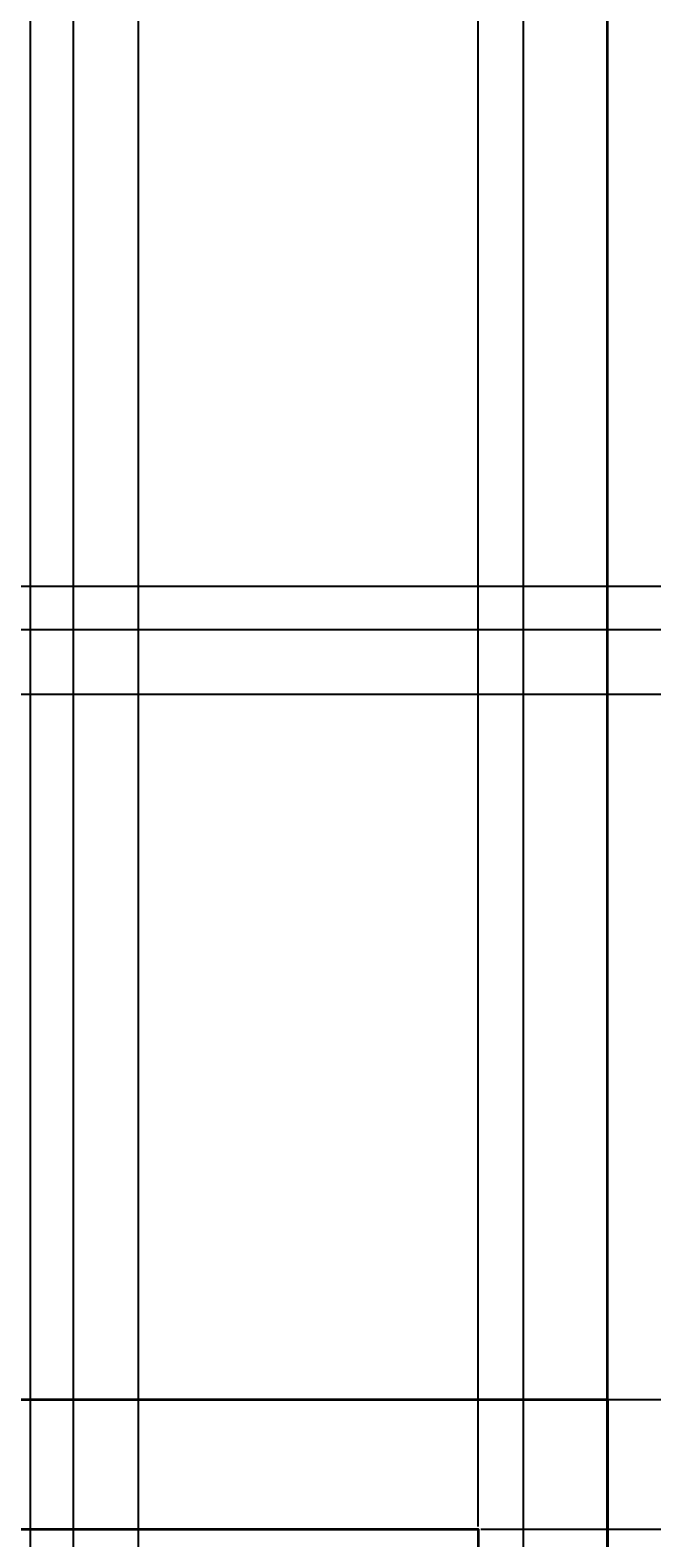
# Model space of a CAD drawing. Units: inches. Extents: x -6 to 289, y -8 to 323.
# Tile 69 of 107: x 234 to 248, y 159 to 194. Entities that reach past the tile are written whole.
import ezdxf

# ---------------------------------------------------------------- set-up
doc = ezdxf.new("R2010")
doc.units = ezdxf.units.IN
doc.header["$MEASUREMENT"] = 0
for name, color, linetype, lineweight in [('A-ANNO-DIMS', 2, 'Continuous', 18), ('A-ELEV', 7, 'Continuous', 35), ('A-GLAZ', 4, 'Continuous', 25)]:
    doc.layers.add(name, color=color, linetype=linetype, lineweight=lineweight)
doc.styles.get("Standard").update_dxf_attribs({"font": 'arial.ttf'})
doc.dimstyles.get("Standard").update_dxf_attribs({"dimtxt": 0.18, "dimasz": 0.18, "dimexe": 0.18, "dimexo": 0.0625, "dimgap": 0.09, "dimtad": 0, "dimtih": 1, "dimtoh": 1, "dimdec": 4, "dimzin": 0, "dimdsep": 46, "dimtxsty": 'Standard', "dimcen": 0.09, "dimadec": 0, "dimazin": 0, "dimtfac": 1, "dimtdec": 4, "dimtofl": 0, "dimtmove": 0, "dimatfit": 3, "dimfxl": 1, "dimtolj": 1, "dimtzin": 0, "dimarcsym": 0})

# ---------------------------------------------------------------- blocks, each defined once
blk = doc.blocks.new('*D14')
at = {"layer": 'A-ANNO-DIMS', "color": 0, "lineweight": -2, "transparency": 16777216}
for p, q in [((236.292, 226.951), (236.292, 322.969)), ((247.164, 162.411), (247.164, 322.969)), ((236.472, 322.789), (241.274, 322.789)), ((246.984, 322.789), (242.182, 322.789))]:
    blk.add_line(p, q, dxfattribs=at)
at = {"layer": 'A-ANNO-DIMS', "color": 0, "transparency": 16777216}
for points in [[(236.472, 322.819), (236.472, 322.759), (236.292, 322.789)], [(246.984, 322.819), (246.984, 322.759), (247.164, 322.789)]]:
    blk.add_solid(points, dxfattribs=at)
at = {"layer": 'Defpoints', "color": 0, "transparency": 16777216}
for p in [(247.164, 322.789), (236.292, 226.889), (247.164, 162.348)]:
    blk.add_point(p, dxfattribs=at)
at = {"layer": 'A-ANNO-DIMS', "color": 0, "transparency": 16777216, "insert": (241.728, 322.789), "char_height": 0.18, "attachment_point": 5}
blk.add_mtext('\\A1;10.872', dxfattribs=at)
blk = doc.blocks.new('*D15')
at = {"layer": 'A-ANNO-DIMS', "color": 0, "lineweight": -2, "transparency": 16777216}
for p, q in [((247.164, 162.411), (247.164, 322.969)), ((271.164, 7.351), (271.164, 322.969)), ((247.344, 322.789), (258.944, 322.789)), ((270.984, 322.789), (259.384, 322.789))]:
    blk.add_line(p, q, dxfattribs=at)
at = {"layer": 'A-ANNO-DIMS', "color": 0, "transparency": 16777216}
for points in [[(247.344, 322.819), (247.344, 322.759), (247.164, 322.789)], [(270.984, 322.819), (270.984, 322.759), (271.164, 322.789)]]:
    blk.add_solid(points, dxfattribs=at)
at = {"layer": 'Defpoints', "color": 0, "transparency": 16777216}
for p in [(271.164, 322.789), (247.164, 162.348), (271.164, 7.289)]:
    blk.add_point(p, dxfattribs=at)
at = {"layer": 'A-ANNO-DIMS', "color": 0, "transparency": 16777216, "insert": (259.164, 322.789), "char_height": 0.18, "attachment_point": 5}
blk.add_mtext('\\A1;24', dxfattribs=at)
blk = doc.blocks.new('*D24')
at = {"layer": 'A-ANNO-DIMS', "color": 0, "lineweight": -2, "transparency": 16777216}
for p, q in [((126.946, 178.654), (288.653, 178.654)), ((288.473, 178.474), (288.473, 159.153)), ((288.473, 139.469), (288.473, 158.789)), ((259.226, 139.289), (288.653, 139.289))]:
    blk.add_line(p, q, dxfattribs=at)
at = {"layer": 'A-ANNO-DIMS', "color": 0, "transparency": 16777216}
for points in [[(288.443, 178.474), (288.503, 178.474), (288.473, 178.654)], [(288.443, 139.469), (288.503, 139.469), (288.473, 139.289)]]:
    blk.add_solid(points, dxfattribs=at)
at = {"layer": 'Defpoints', "color": 0, "transparency": 16777216}
for p in [(126.883, 178.654), (288.473, 178.654), (259.164, 139.289)]:
    blk.add_point(p, dxfattribs=at)
at = {"layer": 'A-ANNO-DIMS', "color": 0, "transparency": 16777216, "insert": (288.473, 158.971), "char_height": 0.18, "attachment_point": 5}
blk.add_mtext('\\A1;39.365', dxfattribs=at)
blk = doc.blocks.new('*D25')
at = {"layer": 'A-ANNO-DIMS', "color": 0, "lineweight": -2, "transparency": 16777216}
for p, q in [((126.946, 226.654), (288.653, 226.654)), ((288.473, 226.474), (288.473, 202.836)), ((288.473, 178.834), (288.473, 202.472)), ((126.946, 178.654), (288.653, 178.654))]:
    blk.add_line(p, q, dxfattribs=at)
at = {"layer": 'A-ANNO-DIMS', "color": 0, "transparency": 16777216}
for points in [[(288.443, 226.474), (288.503, 226.474), (288.473, 226.654)], [(288.443, 178.834), (288.503, 178.834), (288.473, 178.654)]]:
    blk.add_solid(points, dxfattribs=at)
at = {"layer": 'Defpoints', "color": 0, "transparency": 16777216}
for p in [(126.883, 226.654), (288.473, 226.654), (126.883, 178.654)]:
    blk.add_point(p, dxfattribs=at)
at = {"layer": 'A-ANNO-DIMS', "color": 0, "transparency": 16777216, "insert": (288.473, 202.654), "char_height": 0.18, "attachment_point": 5}
blk.add_mtext('\\A1;48', dxfattribs=at)
blk = doc.blocks.new('*D35')
at = {"layer": 'A-ANNO-DIMS', "color": 0, "lineweight": -2, "transparency": 16777216}
for p, q in [((167.446, 180.154), (288.653, 180.154)), ((288.473, 179.974), (288.473, 179.586)), ((288.473, 178.834), (288.473, 179.222)), ((168.946, 178.654), (288.653, 178.654))]:
    blk.add_line(p, q, dxfattribs=at)
at = {"layer": 'A-ANNO-DIMS', "color": 0, "transparency": 16777216}
for points in [[(288.443, 179.974), (288.503, 179.974), (288.473, 180.154)], [(288.443, 178.834), (288.503, 178.834), (288.473, 178.654)]]:
    blk.add_solid(points, dxfattribs=at)
at = {"layer": 'Defpoints', "color": 0, "transparency": 16777216}
for p in [(167.383, 180.154), (288.473, 180.154), (168.883, 178.654)]:
    blk.add_point(p, dxfattribs=at)
at = {"layer": 'A-ANNO-DIMS', "color": 0, "transparency": 16777216, "insert": (288.473, 179.404), "char_height": 0.18, "attachment_point": 5}
blk.add_mtext('\\A1;1.5', dxfattribs=at)
blk = doc.blocks.new('*D36')
at = {"layer": 'A-ANNO-DIMS', "color": 0, "lineweight": -2, "transparency": 16777216}
for p, q in [((166.446, 181.154), (288.653, 181.154)), ((288.473, 180.974), (288.473, 180.834)), ((288.473, 180.334), (288.473, 180.474)), ((167.446, 180.154), (288.653, 180.154))]:
    blk.add_line(p, q, dxfattribs=at)
at = {"layer": 'A-ANNO-DIMS', "color": 0, "transparency": 16777216}
for points in [[(288.443, 180.974), (288.503, 180.974), (288.473, 181.154)], [(288.443, 180.334), (288.503, 180.334), (288.473, 180.154)]]:
    blk.add_solid(points, dxfattribs=at)
at = {"layer": 'Defpoints', "color": 0, "transparency": 16777216}
for p in [(166.383, 181.154), (288.473, 181.154), (167.383, 180.154)]:
    blk.add_point(p, dxfattribs=at)
at = {"layer": 'A-ANNO-DIMS', "color": 0, "transparency": 16777216, "insert": (288.473, 180.654), "char_height": 0.18, "attachment_point": 5}
blk.add_mtext('\\A1;1', dxfattribs=at)
blk = doc.blocks.new('*D37')
at = {"layer": 'A-ANNO-DIMS', "color": 0, "lineweight": -2, "transparency": 16777216}
for p, q in [((166.446, 224.154), (288.653, 224.154)), ((288.473, 223.974), (288.473, 202.836)), ((288.473, 181.334), (288.473, 202.472)), ((166.446, 181.154), (288.653, 181.154))]:
    blk.add_line(p, q, dxfattribs=at)
at = {"layer": 'A-ANNO-DIMS', "color": 0, "transparency": 16777216}
for points in [[(288.443, 223.974), (288.503, 223.974), (288.473, 224.154)], [(288.443, 181.334), (288.503, 181.334), (288.473, 181.154)]]:
    blk.add_solid(points, dxfattribs=at)
at = {"layer": 'Defpoints', "color": 0, "transparency": 16777216}
for p in [(166.383, 224.154), (288.473, 224.154), (166.383, 181.154)]:
    blk.add_point(p, dxfattribs=at)
at = {"layer": 'A-ANNO-DIMS', "color": 0, "transparency": 16777216, "insert": (288.473, 202.654), "char_height": 0.18, "attachment_point": 5}
blk.add_mtext('\\A1;43', dxfattribs=at)
blk = doc.blocks.new('*D44')
at = {"layer": 'A-ANNO-DIMS', "color": 0, "lineweight": -2, "transparency": 16777216}
for p, q in [((212.292, 224.326), (212.292, -8.391)), ((233.792, 224.326), (233.792, -8.391)), ((212.472, -8.211), (222.716, -8.211)), ((233.612, -8.211), (223.368, -8.211))]:
    blk.add_line(p, q, dxfattribs=at)
at = {"layer": 'A-ANNO-DIMS', "color": 0, "transparency": 16777216}
for points in [[(212.472, -8.181), (212.472, -8.241), (212.292, -8.211)], [(233.612, -8.181), (233.612, -8.241), (233.792, -8.211)]]:
    blk.add_solid(points, dxfattribs=at)
at = {"layer": 'Defpoints', "color": 0, "transparency": 16777216}
for p in [(212.292, 224.389), (233.792, 224.389), (233.792, -8.211)]:
    blk.add_point(p, dxfattribs=at)
at = {"layer": 'A-ANNO-DIMS', "color": 0, "transparency": 16777216, "insert": (223.042, -8.211), "char_height": 0.18, "attachment_point": 5}
blk.add_mtext('\\A1;21.5', dxfattribs=at)
blk = doc.blocks.new('*D45')
at = {"layer": 'A-ANNO-DIMS', "color": 0, "lineweight": -2, "transparency": 16777216}
for p, q in [((234.792, 225.326), (234.792, -8.391)), ((233.792, 224.326), (233.792, -8.391)), ((233.972, -8.211), (234.169, -8.211)), ((234.612, -8.211), (234.415, -8.211))]:
    blk.add_line(p, q, dxfattribs=at)
at = {"layer": 'A-ANNO-DIMS', "color": 0, "transparency": 16777216}
for points in [[(233.972, -8.181), (233.972, -8.241), (233.792, -8.211)], [(234.612, -8.181), (234.612, -8.241), (234.792, -8.211)]]:
    blk.add_solid(points, dxfattribs=at)
at = {"layer": 'Defpoints', "color": 0, "transparency": 16777216}
for p in [(234.792, 225.389), (233.792, 224.389), (234.792, -8.211)]:
    blk.add_point(p, dxfattribs=at)
at = {"layer": 'A-ANNO-DIMS', "color": 0, "transparency": 16777216, "insert": (234.292, -8.211), "char_height": 0.18, "attachment_point": 5}
blk.add_mtext('\\A1;1', dxfattribs=at)
blk = doc.blocks.new('*D46')
at = {"layer": 'A-ANNO-DIMS', "color": 0, "lineweight": -2, "transparency": 16777216}
for p, q in [((236.292, 226.826), (236.292, -8.391)), ((234.792, 225.326), (234.792, -8.391)), ((234.972, -8.211), (235.296, -8.211)), ((236.112, -8.211), (235.788, -8.211))]:
    blk.add_line(p, q, dxfattribs=at)
at = {"layer": 'A-ANNO-DIMS', "color": 0, "transparency": 16777216}
for points in [[(234.972, -8.181), (234.972, -8.241), (234.792, -8.211)], [(236.112, -8.181), (236.112, -8.241), (236.292, -8.211)]]:
    blk.add_solid(points, dxfattribs=at)
at = {"layer": 'Defpoints', "color": 0, "transparency": 16777216}
for p in [(236.292, 226.889), (234.792, 225.389), (236.292, -8.211)]:
    blk.add_point(p, dxfattribs=at)
at = {"layer": 'A-ANNO-DIMS', "color": 0, "transparency": 16777216, "insert": (235.542, -8.211), "char_height": 0.18, "attachment_point": 5}
blk.add_mtext('\\A1;1.5', dxfattribs=at)
blk = doc.blocks.new('*D47')
at = {"layer": 'A-ANNO-DIMS', "color": 0, "lineweight": -2, "transparency": 16777216}
for p, q in [((233.854, 224.389), (288.653, 224.389)), ((288.473, 224.209), (288.473, 193.55)), ((288.473, 162.528), (288.473, 193.187)), ((236.354, 162.348), (288.653, 162.348))]:
    blk.add_line(p, q, dxfattribs=at)
at = {"layer": 'A-ANNO-DIMS', "color": 0, "transparency": 16777216}
for points in [[(288.443, 224.209), (288.503, 224.209), (288.473, 224.389)], [(288.443, 162.528), (288.503, 162.528), (288.473, 162.348)]]:
    blk.add_solid(points, dxfattribs=at)
at = {"layer": 'Defpoints', "color": 0, "transparency": 16777216}
for p in [(233.792, 224.389), (288.473, 224.389), (236.292, 162.348)]:
    blk.add_point(p, dxfattribs=at)
at = {"layer": 'A-ANNO-DIMS', "color": 0, "transparency": 16777216, "insert": (288.473, 193.369), "char_height": 0.18, "attachment_point": 5}
blk.add_mtext('\\A1;62.04', dxfattribs=at)
blk = doc.blocks.new('*D81')
at = {"layer": 'A-ANNO-DIMS', "color": 0, "lineweight": -2, "transparency": 16777216}
for p, q in [((230.292, 68.842), (230.292, 322.969)), ((245.215, 66.286), (245.215, 322.969)), ((230.472, 322.789), (237.298, 322.789)), ((245.035, 322.789), (238.208, 322.789))]:
    blk.add_line(p, q, dxfattribs=at)
at = {"layer": 'A-ANNO-DIMS', "color": 0, "transparency": 16777216}
for points in [[(230.472, 322.819), (230.472, 322.759), (230.292, 322.789)], [(245.035, 322.819), (245.035, 322.759), (245.215, 322.789)]]:
    blk.add_solid(points, dxfattribs=at)
at = {"layer": 'Defpoints', "color": 0, "transparency": 16777216}
for p in [(245.215, 322.789), (230.292, 68.779), (245.215, 66.224)]:
    blk.add_point(p, dxfattribs=at)
at = {"layer": 'A-ANNO-DIMS', "color": 0, "transparency": 16777216, "insert": (237.753, 322.789), "char_height": 0.18, "attachment_point": 5}
blk.add_mtext('\\A1;14.923', dxfattribs=at)
blk = doc.blocks.new('*D82')
at = {"layer": 'A-ANNO-DIMS', "color": 0, "lineweight": -2, "transparency": 16777216}
for p, q in [((245.215, 66.286), (245.215, 322.969)), ((272.973, 66.286), (272.973, 322.969)), ((245.395, 322.789), (258.699, 322.789)), ((272.793, 322.789), (259.489, 322.789))]:
    blk.add_line(p, q, dxfattribs=at)
at = {"layer": 'A-ANNO-DIMS', "color": 0, "transparency": 16777216}
for points in [[(245.395, 322.819), (245.395, 322.759), (245.215, 322.789)], [(272.793, 322.819), (272.793, 322.759), (272.973, 322.789)]]:
    blk.add_solid(points, dxfattribs=at)
at = {"layer": 'Defpoints', "color": 0, "transparency": 16777216}
for p in [(272.973, 322.789), (245.215, 66.224), (272.973, 66.224)]:
    blk.add_point(p, dxfattribs=at)
at = {"layer": 'A-ANNO-DIMS', "color": 0, "transparency": 16777216, "insert": (259.094, 322.789), "char_height": 0.18, "attachment_point": 5}
blk.add_mtext('\\A1;27.76', dxfattribs=at)
blk = doc.blocks.new('*D98')
at = {"layer": 'A-ANNO-DIMS', "color": 0, "lineweight": -2, "transparency": 16777216}
for p, q in [((202.741, 159.411), (202.741, 322.969)), ((244.164, 159.411), (244.164, 322.969)), ((202.921, 322.789), (223.056, 322.789)), ((243.984, 322.789), (223.849, 322.789))]:
    blk.add_line(p, q, dxfattribs=at)
at = {"layer": 'A-ANNO-DIMS', "color": 0, "transparency": 16777216}
for points in [[(202.921, 322.819), (202.921, 322.759), (202.741, 322.789)], [(243.984, 322.819), (243.984, 322.759), (244.164, 322.789)]]:
    blk.add_solid(points, dxfattribs=at)
at = {"layer": 'Defpoints', "color": 0, "transparency": 16777216}
for p in [(244.164, 322.789), (202.741, 159.348), (244.164, 159.348)]:
    blk.add_point(p, dxfattribs=at)
at = {"layer": 'A-ANNO-DIMS', "color": 0, "transparency": 16777216, "insert": (223.452, 322.789), "char_height": 0.18, "attachment_point": 5}
blk.add_mtext('\\A1;41.42', dxfattribs=at)
blk = doc.blocks.new('*D99')
at = {"layer": 'A-ANNO-DIMS', "color": 0, "lineweight": -2, "transparency": 16777216}
for p, q in [((244.164, 159.411), (244.164, 322.969)), ((247.164, 162.411), (247.164, 322.969)), ((244.344, 322.789), (245.515, 322.789)), ((246.984, 322.789), (245.813, 322.789))]:
    blk.add_line(p, q, dxfattribs=at)
at = {"layer": 'A-ANNO-DIMS', "color": 0, "transparency": 16777216}
for points in [[(244.344, 322.819), (244.344, 322.759), (244.164, 322.789)], [(246.984, 322.819), (246.984, 322.759), (247.164, 322.789)]]:
    blk.add_solid(points, dxfattribs=at)
at = {"layer": 'Defpoints', "color": 0, "transparency": 16777216}
for p in [(247.164, 322.789), (247.164, 162.348), (244.164, 159.348)]:
    blk.add_point(p, dxfattribs=at)
at = {"layer": 'A-ANNO-DIMS', "color": 0, "transparency": 16777216, "insert": (245.664, 322.789), "char_height": 0.18, "attachment_point": 5}
blk.add_mtext('\\A1;3', dxfattribs=at)
blk = doc.blocks.new('*D100')
at = {"layer": 'A-ANNO-DIMS', "color": 0, "lineweight": -2, "transparency": 16777216}
for p, q in [((247.164, 162.411), (247.164, 322.969)), ((259.164, 139.351), (259.164, 322.969)), ((247.344, 322.789), (252.954, 322.789)), ((258.984, 322.789), (253.373, 322.789))]:
    blk.add_line(p, q, dxfattribs=at)
at = {"layer": 'A-ANNO-DIMS', "color": 0, "transparency": 16777216}
for points in [[(247.344, 322.819), (247.344, 322.759), (247.164, 322.789)], [(258.984, 322.819), (258.984, 322.759), (259.164, 322.789)]]:
    blk.add_solid(points, dxfattribs=at)
at = {"layer": 'Defpoints', "color": 0, "transparency": 16777216}
for p in [(259.164, 322.789), (247.164, 162.348), (259.164, 139.289)]:
    blk.add_point(p, dxfattribs=at)
at = {"layer": 'A-ANNO-DIMS', "color": 0, "transparency": 16777216, "insert": (253.164, 322.789), "char_height": 0.18, "attachment_point": 5}
blk.add_mtext('\\A1;12', dxfattribs=at)
blk = doc.blocks.new('*D103')
at = {"layer": 'A-ANNO-DIMS', "color": 0, "lineweight": -2, "transparency": 16777216}
for p, q in [((244.226, 159.348), (288.653, 159.348)), ((288.473, 159.168), (288.473, 151)), ((288.473, 142.469), (288.473, 150.637)), ((244.226, 142.289), (288.653, 142.289))]:
    blk.add_line(p, q, dxfattribs=at)
at = {"layer": 'A-ANNO-DIMS', "color": 0, "transparency": 16777216}
for points in [[(288.443, 159.168), (288.503, 159.168), (288.473, 159.348)], [(288.443, 142.469), (288.503, 142.469), (288.473, 142.289)]]:
    blk.add_solid(points, dxfattribs=at)
at = {"layer": 'Defpoints', "color": 0, "transparency": 16777216}
for p in [(244.164, 159.348), (288.473, 159.348), (244.164, 142.289)]:
    blk.add_point(p, dxfattribs=at)
at = {"layer": 'A-ANNO-DIMS', "color": 0, "transparency": 16777216, "insert": (288.473, 150.819), "char_height": 0.18, "attachment_point": 5}
blk.add_mtext('\\A1;17.06', dxfattribs=at)
blk = doc.blocks.new('*D104')
at = {"layer": 'A-ANNO-DIMS', "color": 0, "lineweight": -2, "transparency": 16777216}
for p, q in [((247.226, 162.348), (288.653, 162.348)), ((288.473, 162.168), (288.473, 161.03)), ((288.473, 159.528), (288.473, 160.666)), ((244.226, 159.348), (288.653, 159.348))]:
    blk.add_line(p, q, dxfattribs=at)
at = {"layer": 'A-ANNO-DIMS', "color": 0, "transparency": 16777216}
for points in [[(288.443, 162.168), (288.503, 162.168), (288.473, 162.348)], [(288.443, 159.528), (288.503, 159.528), (288.473, 159.348)]]:
    blk.add_solid(points, dxfattribs=at)
at = {"layer": 'Defpoints', "color": 0, "transparency": 16777216}
for p in [(247.164, 162.348), (288.473, 162.348), (244.164, 159.348)]:
    blk.add_point(p, dxfattribs=at)
at = {"layer": 'A-ANNO-DIMS', "color": 0, "transparency": 16777216, "insert": (288.473, 160.848), "char_height": 0.18, "attachment_point": 5}
blk.add_mtext('\\A1;3', dxfattribs=at)

msp = doc.modelspace()

# ---------------------------------------------------------------- linework, layer by layer
at = {"layer": 'A-ELEV'}
msp.add_line((247.1638, 139.2888), (247.1638, 247.2888), dxfattribs=at)
for points in [[(247.1638, 139.2888), (115.1638, 139.2888), (115.1638, 162.3484), (247.1638, 162.3484)], [(244.1638, 142.2888), (118.1638, 142.2888), (118.1638, 159.3484), (244.1638, 159.3484)]]:
    msp.add_lwpolyline(points, close=True, dxfattribs=at)
at = {"layer": 'A-GLAZ'}
msp.add_line((234.7918, 225.3887), (234.7918, 162.3484), dxfattribs=at)
msp.add_lwpolyline([(188.2918, 162.3484), (188.2918, 226.8887), (236.2918, 226.8887), (236.2918, 162.3484)], dxfattribs=at)

# ---------------------------------------------------------------- dimensions: what is measured, and where the dimension line sits
at = {"layer": 'A-ANNO-DIMS'}
for base, p1, p2, override, picture, middle in [((244.1638, 322.7888), (202.741, 159.3484), (244.1638, 159.3484), {"dimdec": 2, "dimlfac": 1, "dimrnd": 0, "dimzin": 0, "dimdsep": 46, "dimlunit": 2}, '*D98', (223.4524, 322.7888)), ((245.2146, 322.7888), (230.2918, 68.7795), (245.2146, 66.2238), {"dimdec": 3, "dimlfac": 1, "dimrnd": 0, "dimzin": 0, "dimdsep": 46, "dimlunit": 2}, '*D81', (237.7532, 322.7888)), ((247.1638, 322.7888), (236.2918, 226.8887), (247.1638, 162.3484), {"dimdec": 3, "dimlfac": 1, "dimrnd": 0, "dimzin": 0, "dimdsep": 46, "dimlunit": 2}, '*D14', (241.7278, 322.7888)), ((247.1638, 322.7888), (244.1638, 159.3484), (247.1638, 162.3484), {"dimdec": 0, "dimlfac": 1, "dimrnd": 0, "dimzin": 0, "dimdsep": 46, "dimlunit": 2}, '*D99', (245.6638, 322.7888)), ((272.9733, 322.7888), (245.2146, 66.2238), (272.9733, 66.2238), {"dimdec": 2, "dimlfac": 1, "dimrnd": 0, "dimzin": 0, "dimdsep": 46, "dimlunit": 2}, '*D82', (259.0939, 322.7888)), ((271.1638, 322.7888), (247.1638, 162.3484), (271.1638, 7.2888), {"dimdec": 0, "dimlfac": 1, "dimrnd": 0, "dimzin": 0, "dimdsep": 46, "dimlunit": 2}, '*D15', (259.1638, 322.7888)), ((259.1638, 322.7888), (247.1638, 162.3484), (259.1638, 139.2888), {"dimdec": 0, "dimlfac": 1, "dimrnd": 0, "dimzin": 0, "dimdsep": 46, "dimlunit": 2}, '*D100', (253.1638, 322.7888)), ((236.2918, -8.2112), (234.7918, 225.3887), (236.2918, 226.8887), {"dimdec": 1, "dimlfac": 1, "dimrnd": 0, "dimzin": 0, "dimdsep": 46, "dimlunit": 2}, '*D46', (235.5418, -8.2112)), ((234.7918, -8.2112), (233.7918, 224.3887), (234.7918, 225.3887), {"dimdec": 0, "dimlfac": 1, "dimrnd": 0, "dimzin": 0, "dimdsep": 46, "dimlunit": 2}, '*D45', (234.2918, -8.2112)), ((233.7918, -8.2112), (212.2918, 224.3887), (233.7918, 224.3887), {"dimdec": 1, "dimlfac": 1, "dimrnd": 0, "dimzin": 0, "dimdsep": 46, "dimlunit": 2}, '*D44', (223.0418, -8.2112))]:
    dim = msp.add_linear_dim(base=base, p1=p1, p2=p2, dimstyle='Standard', override=override, dxfattribs=at)
    dim.commit()
    dim.dimension.update_dxf_attribs({"geometry": picture, "text_midpoint": middle})
for base, p1, p2, override, picture, middle in [((288.4733, 226.654), (126.8835, 178.654), (126.8835, 226.654), {"dimdec": 0, "dimlfac": 1, "dimrnd": 0, "dimzin": 0, "dimdsep": 46, "dimlunit": 2}, '*D25', (288.4733, 202.654)), ((288.4733, 224.3887), (236.2918, 162.3484), (233.7918, 224.3887), {"dimdec": 2, "dimlfac": 1, "dimrnd": 0, "dimzin": 0, "dimdsep": 46, "dimlunit": 2}, '*D47', (288.4733, 193.3685)), ((288.4733, 224.154), (166.3835, 181.154), (166.3835, 224.154), {"dimdec": 0, "dimlfac": 1, "dimrnd": 0, "dimzin": 0, "dimdsep": 46, "dimlunit": 2}, '*D37', (288.4733, 202.654)), ((288.4733, 181.154), (167.3835, 180.154), (166.3835, 181.154), {"dimdec": 0, "dimlfac": 1, "dimrnd": 0, "dimzin": 0, "dimdsep": 46, "dimlunit": 2}, '*D36', (288.4733, 180.654)), ((288.4733, 180.154), (168.8835, 178.654), (167.3835, 180.154), {"dimdec": 1, "dimlfac": 1, "dimrnd": 0, "dimzin": 0, "dimdsep": 46, "dimlunit": 2}, '*D35', (288.4733, 179.404)), ((288.4733, 178.654), (259.1638, 139.2888), (126.8835, 178.654), {"dimdec": 3, "dimlfac": 1, "dimrnd": 0, "dimzin": 0, "dimdsep": 46, "dimlunit": 2}, '*D24', (288.4733, 158.9714)), ((288.4733, 162.3484), (244.1638, 159.3484), (247.1638, 162.3484), {"dimdec": 0, "dimlfac": 1, "dimrnd": 0, "dimzin": 0, "dimdsep": 46, "dimlunit": 2}, '*D104', (288.4733, 160.8484)), ((288.4733, 159.3484), (244.1638, 142.2888), (244.1638, 159.3484), {"dimdec": 2, "dimlfac": 1, "dimrnd": 0, "dimzin": 0, "dimdsep": 46, "dimlunit": 2}, '*D103', (288.4733, 150.8186))]:
    dim = msp.add_linear_dim(base=base, p1=p1, p2=p2, angle=90, dimstyle='Standard', override=override, dxfattribs=at)
    dim.commit()
    dim.dimension.update_dxf_attribs({"geometry": picture, "text_midpoint": middle})

doc.saveas('drawing.dxf')
